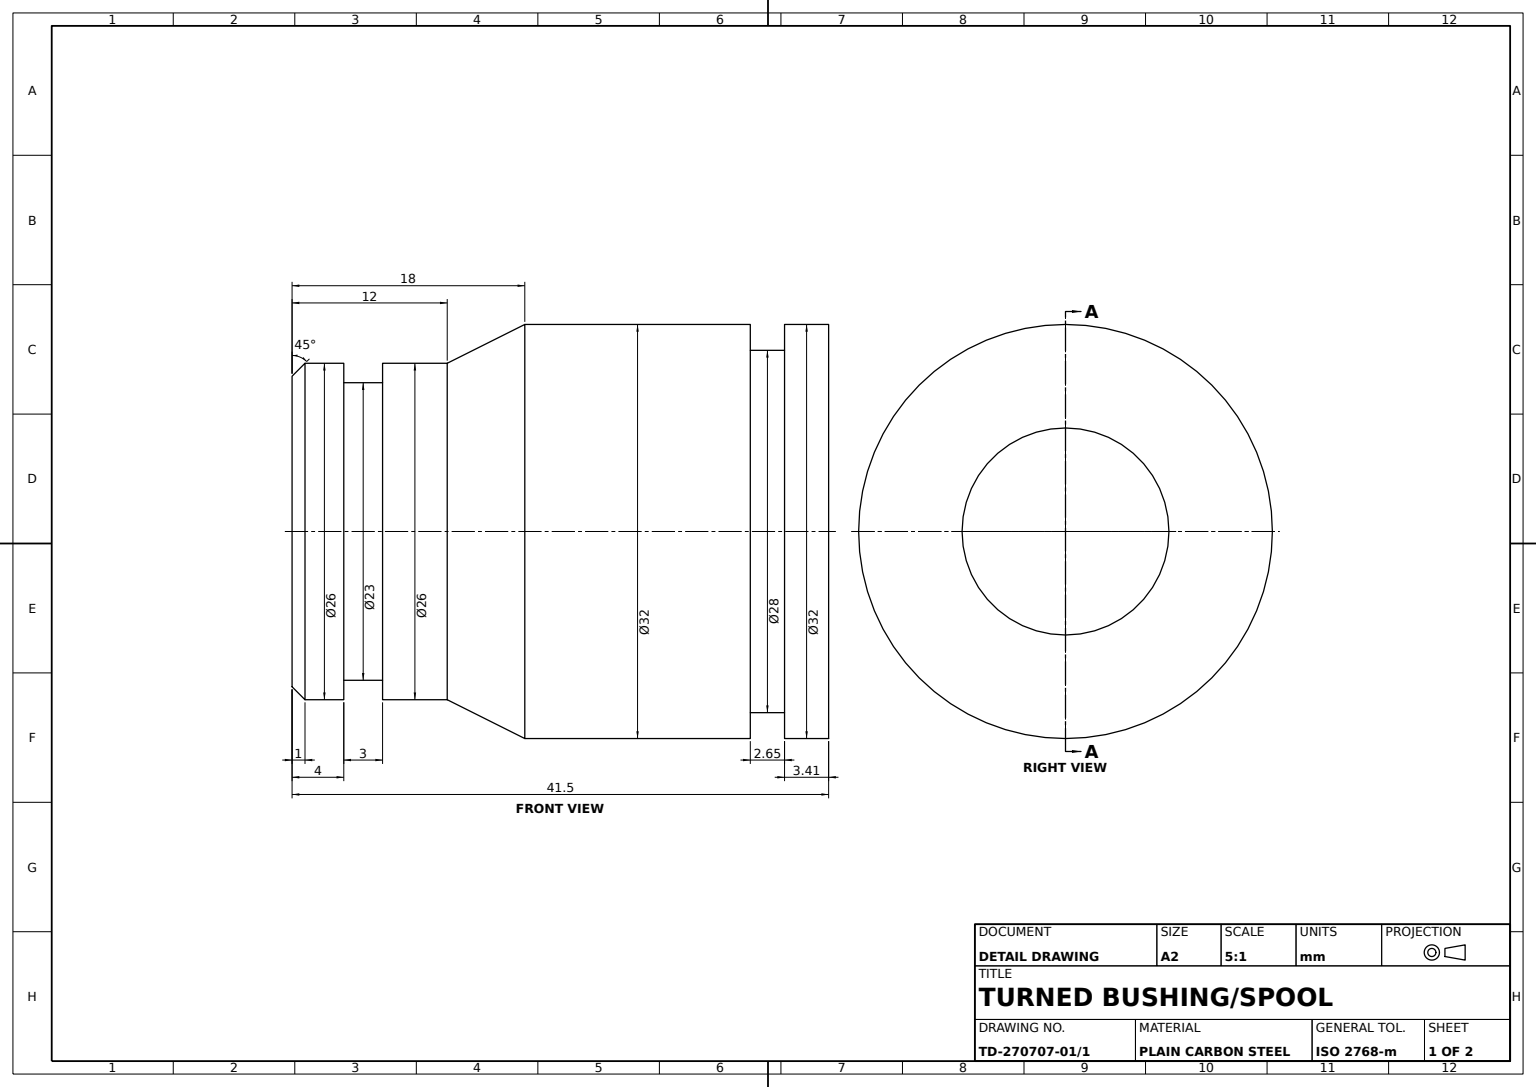
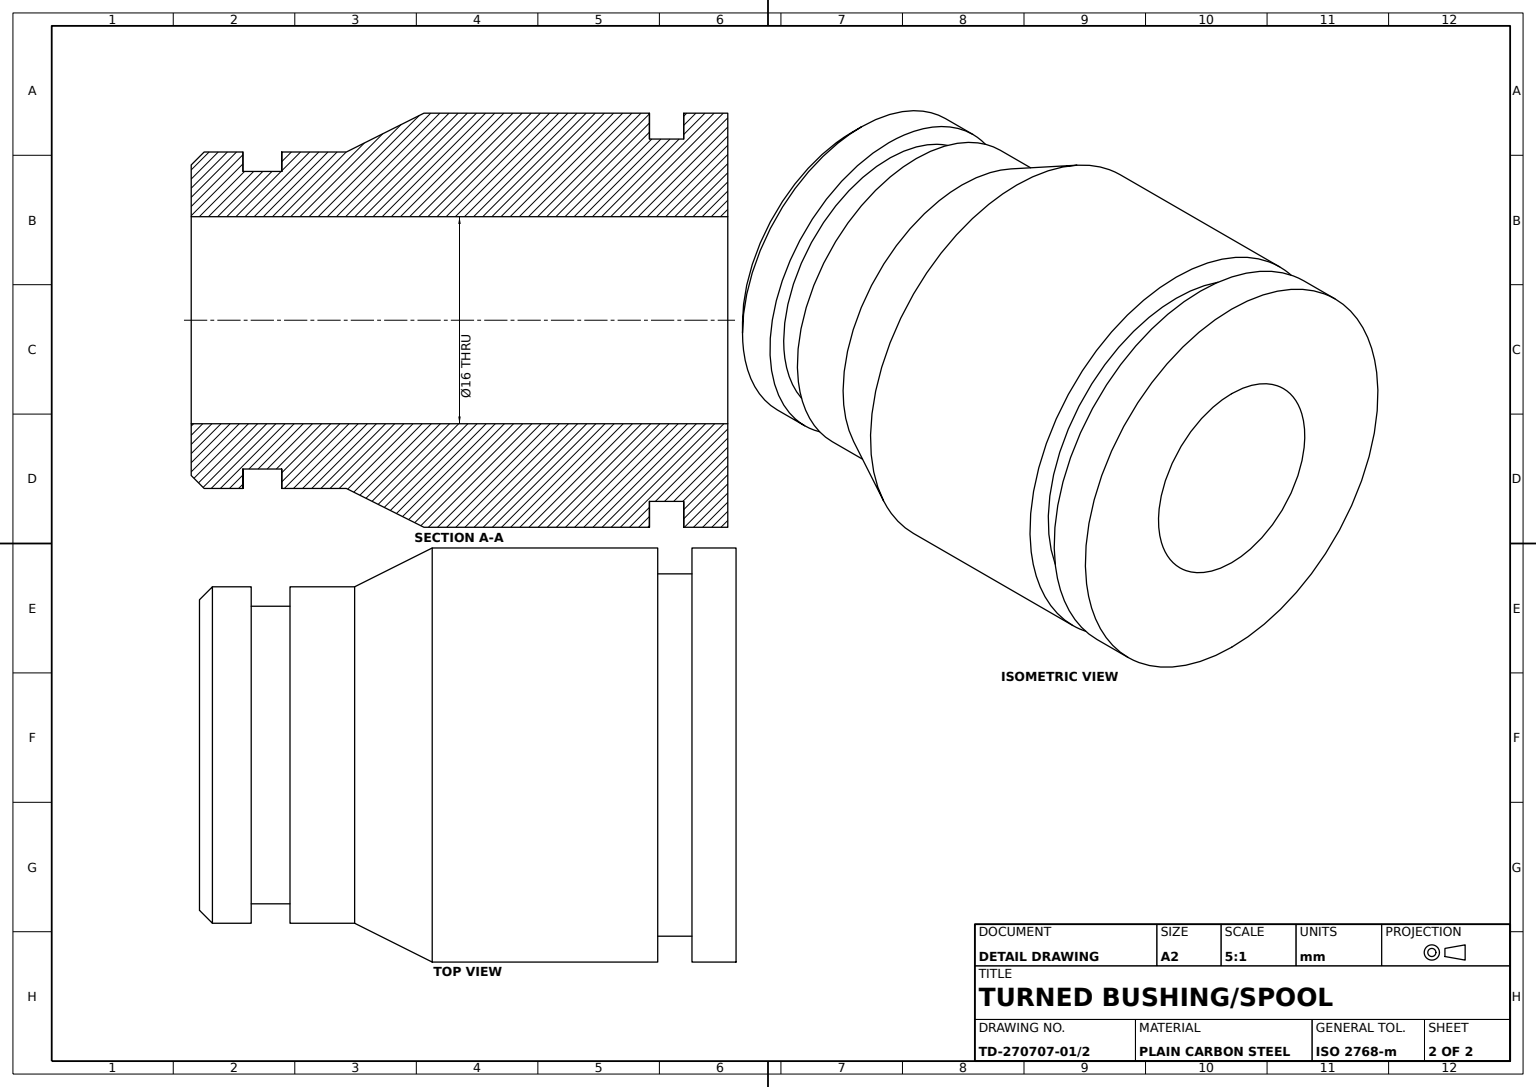
from build123d import *

# Parameters (mm, degrees)
GROOVE_PROFILE_SKETCH_3X3_W = 3
GROOVE_PROFILE_SKETCH_3X3_H = 4.04600801


with BuildPart() as part:
    # Bushing Profile Sketch → Bushing Body Revolve (revolve)
    with BuildSketch(Plane.XY, mode=Mode.PRIVATE) as bushing_body_revolve_sk:
        Polygon((-9.597352736, 8), (31.902647264, 8), (31.902647264, 16), (28.493054394, 16), (28.493054394, 14), (25.843857713, 14), (25.843857713, 16), (8.402647264, 16), (2.402647264, 13), (-8.597352736, 13), (-9.597352736, 12), align=None)
    revolve(bushing_body_revolve_sk.sketch.rotate(Axis((-43.791817978, 0, 0), (1, 0, 0)), 180), axis=Axis((-43.791817978, 0, 0), (1, 0, 0)))

    # Groove Profile Sketch 3x3 → Groove Cut 3x3 (revolve, cut)
    with BuildSketch(Plane.XY, mode=Mode.PRIVATE) as groove_cut_3x3_sk:
        with Locations((-4.097352736, 13.5210982)):
            Rectangle(GROOVE_PROFILE_SKETCH_3X3_W, GROOVE_PROFILE_SKETCH_3X3_H)
    revolve(groove_cut_3x3_sk.sketch.rotate(Axis((-18.397733025, 0, 0), (1, 0, 0)), 180), axis=Axis((-18.397733025, 0, 0), (1, 0, 0)), mode=Mode.SUBTRACT)


solid = part.part
